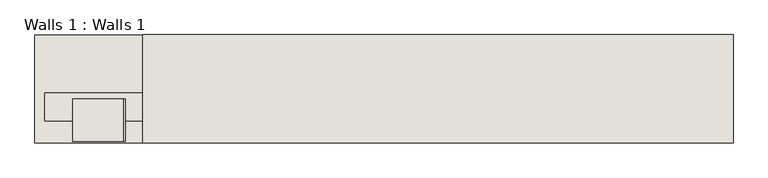
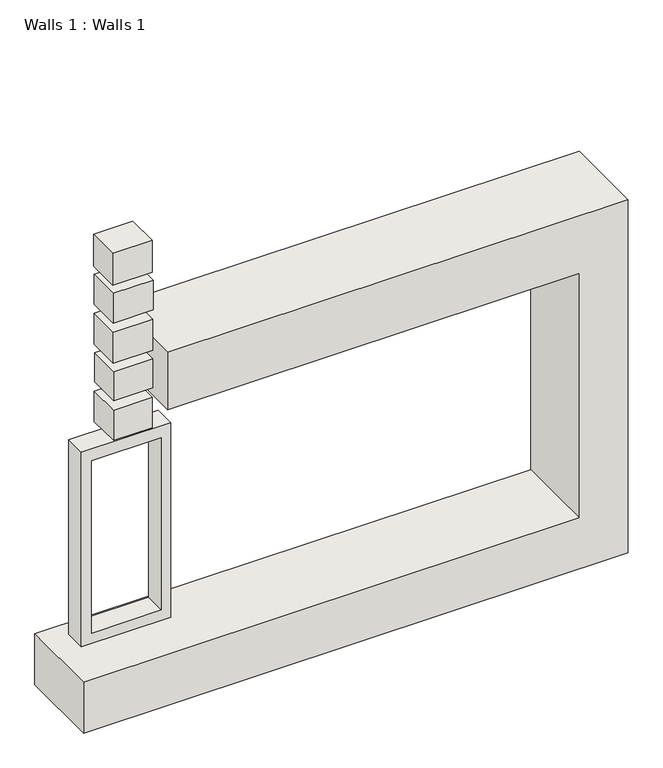
"""IFC4 building model written with IfcOpenShell, lengths in millimetres: wall geometry, Walls 1 : Walls 1."""

from ifc_helpers import new_model, si_unit, frame, origin, place, context, project, spatial, polyline, outline, extrude, source, transform, mapped, element, save


def walls_1_walls_1_66469eba(model_context):
    return source(origin(), model_context, "Body", "SweptSolid", [
        extrude(outline(polyline([(6512.6251814, -6163.3682708), (6512.6251814, -7272.3083357), (3962.4, -7272.3083357), (3962.4, -6163.3682708), (6512.6251814, -6163.3682708)]), holes=[polyline([(6360.2251814, -6281.7083357), (4099.6251814, -6281.7083357), (4099.6251814, -7145.3083357), (6360.2251814, -7145.3083357), (6360.2251814, -6281.7083357)])]), frame((0.0, -2901.4387205, 0.0), z_axis=(0.0, 1.0, 0.0), x_axis=(0.0, 0.0, 1.0)), (0.0, 0.0, 1.0), 272.9870857),
        extrude(outline(polyline([(-6509.4705279, -3096.2997374), (-6999.1814128, -3096.2997374), (-6999.1814128, -2686.826099), (-6509.4705279, -2686.826099), (-6509.4705279, -3096.2997374)])), frame((0.0, 0.0, 8725.9700556), z_axis=(0.0, 0.0, 1.0), x_axis=(1.0, 0.0, 0.0)), (0.0, 0.0, 1.0), 421.4068238),
        extrude(outline(polyline([(-6501.4626173, -3096.2997374), (-6988.2106934, -3096.2997374), (-6988.2106934, -2686.826099), (-6501.4626173, -2686.826099), (-6501.4626173, -3096.2997374)])), frame((0.0, 0.0, 7703.1339675), z_axis=(0.0, 0.0, 1.0), x_axis=(1.0, 0.0, 0.0)), (0.0, 0.0, 1.0), 405.7738967),
        extrude(outline(polyline([(-6507.1507402, -3096.2997374), (-6987.5097206, -3096.2997374), (-6987.5097206, -2686.826099), (-6507.1507402, -2686.826099), (-6507.1507402, -3096.2997374)])), frame((0.0, 0.0, 6687.8447645), z_axis=(0.0, 0.0, 1.0), x_axis=(1.0, 0.0, 0.0)), (0.0, 0.0, 1.0), 399.1428549),
        extrude(outline(polyline([(-6493.5882407, -3096.2997374), (-6991.1494172, -3096.2997374), (-6991.1494172, -2686.826099), (-6493.5882407, -2686.826099), (-6493.5882407, -3096.2997374)])), frame((0.0, 0.0, 8226.5573027), z_axis=(0.0, 0.0, 1.0), x_axis=(1.0, 0.0, 0.0)), (0.0, 0.0, 1.0), 391.3677229),
        extrude(outline(polyline([(-6499.8498202, -3096.2997374), (-6985.2604809, -3096.2997374), (-6985.2604809, -2686.826099), (-6499.8498202, -2686.826099), (-6499.8498202, -3096.2997374)])), frame((0.0, 0.0, 7206.9610058), z_axis=(0.0, 0.0, 1.0), x_axis=(1.0, 0.0, 0.0)), (0.0, 0.0, 1.0), 383.8044816),
        extrude(outline(polyline([(3657.6, -1209.8787413), (3657.6, -7366.6932708), (2991.9319082, -7366.6932708), (2991.9319082, -610.2932708), (3657.6, -610.2932708), (6867.5695878, -610.2932708), (7620.0, -610.2932708), (7620.0, -6325.2932708), (6867.5695878, -6325.2932708), (6867.5695878, -1209.8787413), (3657.6, -1209.8787413)])), frame((0.0, -3110.3864146, 0.0), z_axis=(0.0, 1.0, 0.0), x_axis=(0.0, 0.0, 1.0)), (0.0, 0.0, 1.0), 1045.8603156),
    ])


if __name__ == "__main__":
    model = new_model("IFC4")
    model_context = context("Model", 3, world=origin())
    ifc_project = project(units=[si_unit("LENGTHUNIT", "METRE", prefix="MILLI")], contexts=[model_context])
    site = spatial("IfcSite", under=ifc_project)
    building = spatial("IfcBuilding", under=site)
    placement = place(None, origin())
    walls_1_walls_1_shape = walls_1_walls_1_66469eba(model_context)
    element("IfcWall", 1, ObjectType="Walls 1 : Walls 1", at=placement, inside=building, context=model_context, shape_type="MappedRepresentation", body=[
        mapped(walls_1_walls_1_shape, transform((0.0, 0.0, 0.0), x_axis=(1.0, 0.0, 0.0), y_axis=(0.0, 1.0, 0.0), z_axis=(0.0, 0.0, 1.0))),
    ])
    save(model, "model.ifc")

# Revit data of these elements
# Element 1 (IfcWall, "Walls 1 : Walls 1")
#   Materials on its faces: "Default Wall"
# Materials
#   "Default Wall": colour RGB 128 128 128, transparency 0
